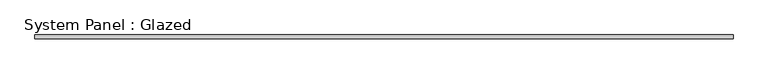
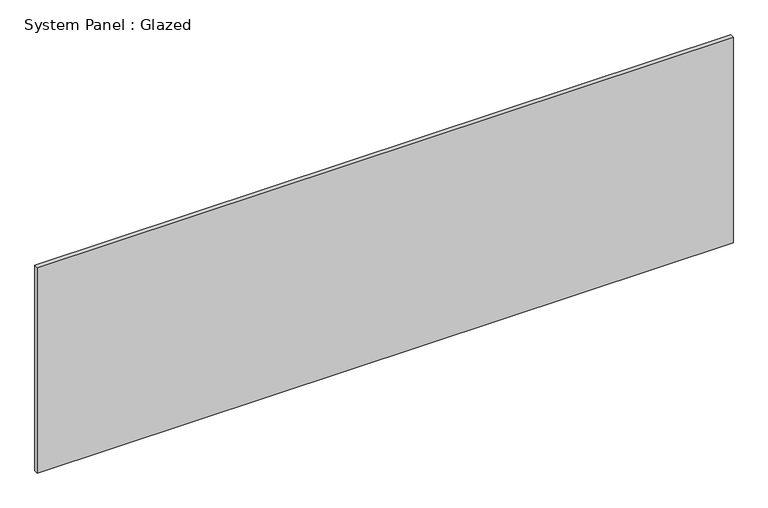
"""IFC4 building model written with IfcOpenShell, lengths in millimetres: plate geometry, System Panel : Glazed."""

from ifc_helpers import new_model, si_unit, origin, origin_with_axes, place, context, project, spatial, polyline, outline, extrude, source, transform, mapped, element, save


def system_panel_glazed_b34c6f43(model_context):
    return source(origin(), model_context, "Body", "SweptSolid", [
        extrude(outline(polyline([(2339.975, 19.05), (-2339.975, 19.05), (-2339.975, 44.45), (2339.975, 44.45), (2339.975, 19.05)])), origin_with_axes(), (0.0, 0.0, 1.0), 1460.5),
    ])


if __name__ == "__main__":
    model = new_model("IFC4")
    model_context = context("Model", 3, world=origin())
    ifc_project = project(units=[si_unit("LENGTHUNIT", "METRE", prefix="MILLI")], contexts=[model_context])
    site = spatial("IfcSite", under=ifc_project)
    building = spatial("IfcBuilding", under=site)
    placement = place(None, origin())
    system_panel_glazed_shape = system_panel_glazed_b34c6f43(model_context)
    element("IfcPlate", 1, ObjectType="System Panel : Glazed", at=placement, inside=building, context=model_context, shape_type="MappedRepresentation", body=[
        mapped(system_panel_glazed_shape, transform((0.0, 0.0, 0.0), x_axis=(1.0, 0.0, 0.0), y_axis=(0.0, 1.0, 0.0), z_axis=(0.0, 0.0, 1.0))),
    ])
    save(model, "model.ifc")

# Revit data of these elements
# Type "System Panel : Glazed"
#   Construction Type Id = "GSP4R"
#   Analytic Construction = "1/8 in Pilkington single glazing"
#   Visual Light Transmittance = 0.9
#   Solar Heat Gain Coefficient = 0.86
#   Heat Transfer Coefficient (U) = 1.18115 BTU/(h·ft²·°F)
# Element 1 (IfcPlate, "System Panel : Glazed")
#   Materials on its faces: "Glass"
# Materials
#   "Glass": class "Glass", colour RGB 0 128 192, transparency 0.75, Description = "Soda Lime Glass", Cost = 0
